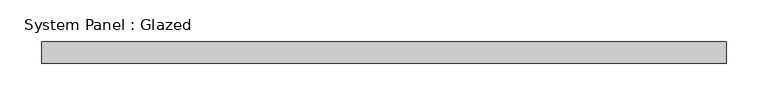
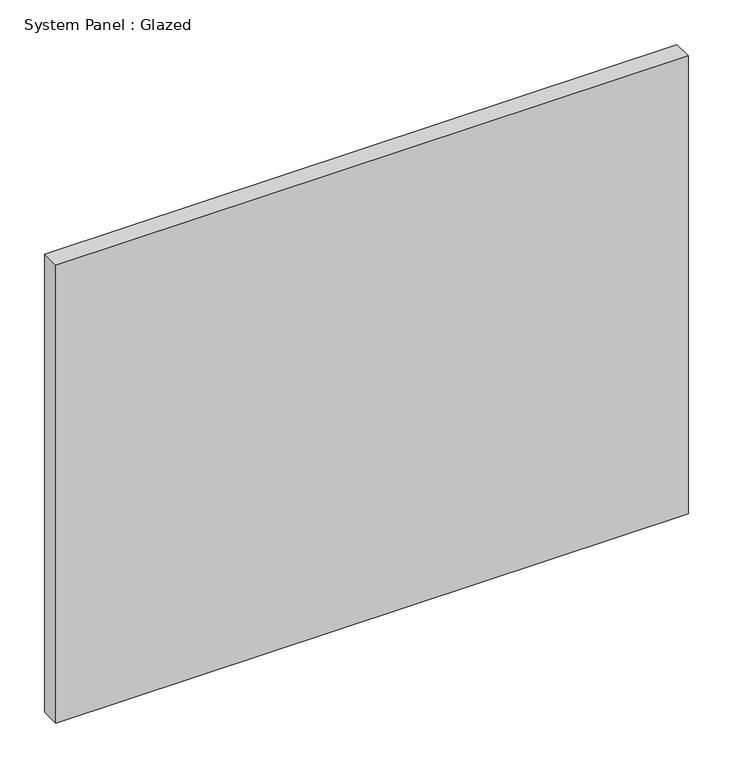
"""IFC4 building model written with IfcOpenShell, lengths in millimetres: plate geometry, System Panel : Glazed."""

from ifc_helpers import new_model, si_unit, origin, origin_with_axes, place, context, project, spatial, polyline, outline, extrude, source, transform, mapped, element, save


def system_panel_glazed_f6fef574(model_context):
    return source(origin(), model_context, "Body", "SweptSolid", [
        extrude(outline(polyline([(409.575, 19.05), (-409.575, 19.05), (-409.575, 44.45), (409.575, 44.45), (409.575, 19.05)])), origin_with_axes(), (0.0, 0.0, 1.0), 627.1281505),
    ])


if __name__ == "__main__":
    model = new_model("IFC4")
    model_context = context("Model", 3, world=origin())
    ifc_project = project(units=[si_unit("LENGTHUNIT", "METRE", prefix="MILLI")], contexts=[model_context])
    site = spatial("IfcSite", under=ifc_project)
    building = spatial("IfcBuilding", under=site)
    placement = place(None, origin())
    system_panel_glazed_shape = system_panel_glazed_f6fef574(model_context)
    element("IfcPlate", 1, ObjectType="System Panel : Glazed", at=placement, inside=building, context=model_context, shape_type="MappedRepresentation", body=[
        mapped(system_panel_glazed_shape, transform((0.0, 0.0, 0.0), x_axis=(1.0, 0.0, 0.0), y_axis=(0.0, 1.0, 0.0), z_axis=(0.0, 0.0, 1.0))),
    ])
    save(model, "model.ifc")

# Revit data of these elements
# Type "System Panel : Glazed"
#   Construction Type Id = "GSP4R"
#   Analytic Construction = "1/8 in Pilkington single glazing"
#   Visual Light Transmittance = 0.9
#   Solar Heat Gain Coefficient = 0.86
#   Heat Transfer Coefficient (U) = 1.18115 BTU/(h·ft²·°F)
#   Define Thermal Properties by = 1
# Element 1 (IfcPlate, "System Panel : Glazed")
#   Materials on its faces: "Glass"
# Materials
#   "Glass": class "Glass", colour RGB 0 128 192, transparency 0.75, Description = "Soda Lime Glass", Cost = 0
